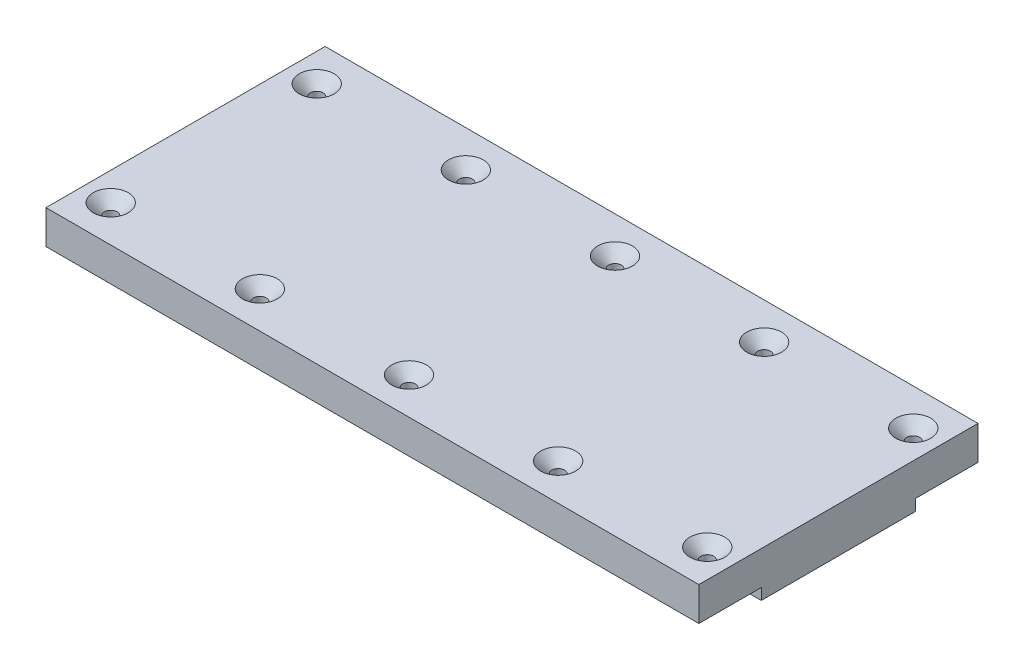
ISO-10303-21;
HEADER;
FILE_DESCRIPTION(('STEP AP214'),'2;1');
FILE_NAME('part.step','',(''),(''),'','','');
FILE_SCHEMA(('AUTOMOTIVE_DESIGN { 1 0 10303 214 1 1 1 1 }'));
ENDSEC;
DATA;
#1=APPLICATION_CONTEXT('core data for automotive mechanical design processes');
#2=APPLICATION_PROTOCOL_DEFINITION('international standard','automotive_design',2000,#1);
#3=PRODUCT_CONTEXT('',#1,'mechanical');
#4=PRODUCT('Part','Part','',(#3));
#5=PRODUCT_RELATED_PRODUCT_CATEGORY('part','',(#4));
#6=PRODUCT_DEFINITION_FORMATION('','',#4);
#7=PRODUCT_DEFINITION_CONTEXT('part definition',#1,'design');
#8=PRODUCT_DEFINITION('design','',#6,#7);
#9=PRODUCT_DEFINITION_SHAPE('','',#8);
#10=(LENGTH_UNIT() NAMED_UNIT(*) SI_UNIT(.MILLI.,.METRE.));
#11=(NAMED_UNIT(*) PLANE_ANGLE_UNIT() SI_UNIT($,.RADIAN.));
#12=(NAMED_UNIT(*) SI_UNIT($,.STERADIAN.) SOLID_ANGLE_UNIT());
#13=UNCERTAINTY_MEASURE_WITH_UNIT(LENGTH_MEASURE(1.E-05),#10,'distance_accuracy_value','');
#14=(GEOMETRIC_REPRESENTATION_CONTEXT(3) GLOBAL_UNCERTAINTY_ASSIGNED_CONTEXT((#13)) GLOBAL_UNIT_ASSIGNED_CONTEXT((#10,
#11,#12)) REPRESENTATION_CONTEXT('',''));
#15=CARTESIAN_POINT('',(0.,0.,0.));
#16=DIRECTION('',(0.,0.,1.));
#17=DIRECTION('',(1.,0.,0.));
#18=AXIS2_PLACEMENT_3D('',#15,#16,#17);
#19=CARTESIAN_POINT('',(580.,10.,68.5));
#20=DIRECTION('',(0.,0.,-1.));
#21=DIRECTION('',(-1.,0.,0.));
#22=AXIS2_PLACEMENT_3D('',#19,#20,#21);
#23=PLANE('',#22);
#24=DIRECTION('',(0.,-1.,0.));
#25=VECTOR('',#24,1.);
#26=CARTESIAN_POINT('',(0.,10.,68.5));
#27=LINE('',#26,#25);
#28=CARTESIAN_POINT('',(0.,10.,68.5));
#29=VERTEX_POINT('',#28);
#30=CARTESIAN_POINT('',(0.,0.,68.5));
#31=VERTEX_POINT('',#30);
#32=EDGE_CURVE('E137',#29,#31,#27,.T.);
#33=ORIENTED_EDGE('',*,*,#32,.T.);
#34=DIRECTION('',(-1.,0.,0.));
#35=VECTOR('',#34,1.);
#36=CARTESIAN_POINT('',(580.,0.,68.5));
#37=LINE('',#36,#35);
#38=CARTESIAN_POINT('',(580.,0.,68.5));
#39=VERTEX_POINT('',#38);
#40=EDGE_CURVE('E169',#39,#31,#37,.T.);
#41=ORIENTED_EDGE('',*,*,#40,.F.);
#42=DIRECTION('',(0.,-1.,0.));
#43=VECTOR('',#42,1.);
#44=CARTESIAN_POINT('',(580.,10.,68.5));
#45=LINE('',#44,#43);
#46=CARTESIAN_POINT('',(580.,10.,68.5));
#47=VERTEX_POINT('',#46);
#48=EDGE_CURVE('E154',#47,#39,#45,.T.);
#49=ORIENTED_EDGE('',*,*,#48,.F.);
#50=DIRECTION('',(-1.,0.,0.));
#51=VECTOR('',#50,1.);
#52=CARTESIAN_POINT('',(580.,10.,68.5));
#53=LINE('',#52,#51);
#54=EDGE_CURVE('E138',#47,#29,#53,.T.);
#55=ORIENTED_EDGE('',*,*,#54,.T.);
#56=EDGE_LOOP('',(#33,#41,#49,#55));
#57=FACE_BOUND('',#56,.T.);
#58=ADVANCED_FACE('F41',(#57),#23,.F.);
#59=CARTESIAN_POINT('',(580.,0.,68.5));
#60=DIRECTION('',(0.,1.,0.));
#61=DIRECTION('',(0.,0.,1.));
#62=AXIS2_PLACEMENT_3D('',#59,#60,#61);
#63=PLANE('',#62);
#64=DIRECTION('',(0.,0.,-1.));
#65=VECTOR('',#64,1.);
#66=CARTESIAN_POINT('',(0.,0.,68.5));
#67=LINE('',#66,#65);
#68=CARTESIAN_POINT('',(0.,0.,-68.5));
#69=VERTEX_POINT('',#68);
#70=EDGE_CURVE('E141',#31,#69,#67,.T.);
#71=ORIENTED_EDGE('',*,*,#70,.T.);
#72=DIRECTION('',(-1.,0.,0.));
#73=VECTOR('',#72,1.);
#74=CARTESIAN_POINT('',(580.,0.,-68.5));
#75=LINE('',#74,#73);
#76=CARTESIAN_POINT('',(580.,0.,-68.5));
#77=VERTEX_POINT('',#76);
#78=EDGE_CURVE('E164',#77,#69,#75,.T.);
#79=ORIENTED_EDGE('',*,*,#78,.F.);
#80=DIRECTION('',(0.,0.,-1.));
#81=VECTOR('',#80,1.);
#82=CARTESIAN_POINT('',(580.,0.,68.5));
#83=LINE('',#82,#81);
#84=EDGE_CURVE('E103',#39,#77,#83,.T.);
#85=ORIENTED_EDGE('',*,*,#84,.F.);
#86=ORIENTED_EDGE('',*,*,#40,.T.);
#87=EDGE_LOOP('',(#71,#79,#85,#86));
#88=FACE_BOUND('',#87,.T.);
#89=ADVANCED_FACE('F257',(#88),#63,.F.);
#90=CARTESIAN_POINT('',(580.,0.,-68.5));
#91=DIRECTION('',(0.,0.,1.));
#92=DIRECTION('',(1.,0.,0.));
#93=AXIS2_PLACEMENT_3D('',#90,#91,#92);
#94=PLANE('',#93);
#95=DIRECTION('',(0.,1.,0.));
#96=VECTOR('',#95,1.);
#97=CARTESIAN_POINT('',(0.,0.,-68.5));
#98=LINE('',#97,#96);
#99=CARTESIAN_POINT('',(0.,10.,-68.5));
#100=VERTEX_POINT('',#99);
#101=EDGE_CURVE('E148',#69,#100,#98,.T.);
#102=ORIENTED_EDGE('',*,*,#101,.T.);
#103=DIRECTION('',(-1.,0.,0.));
#104=VECTOR('',#103,1.);
#105=CARTESIAN_POINT('',(580.,10.,-68.5));
#106=LINE('',#105,#104);
#107=CARTESIAN_POINT('',(580.,10.,-68.5));
#108=VERTEX_POINT('',#107);
#109=EDGE_CURVE('E165',#108,#100,#106,.T.);
#110=ORIENTED_EDGE('',*,*,#109,.F.);
#111=DIRECTION('',(0.,1.,0.));
#112=VECTOR('',#111,1.);
#113=CARTESIAN_POINT('',(580.,0.,-68.5));
#114=LINE('',#113,#112);
#115=EDGE_CURVE('E351',#77,#108,#114,.T.);
#116=ORIENTED_EDGE('',*,*,#115,.F.);
#117=ORIENTED_EDGE('',*,*,#78,.T.);
#118=EDGE_LOOP('',(#102,#110,#116,#117));
#119=FACE_BOUND('',#118,.T.);
#120=ADVANCED_FACE('F266',(#119),#94,.F.);
#121=CARTESIAN_POINT('',(580.,10.,-68.5));
#122=DIRECTION('',(0.,1.,0.));
#123=DIRECTION('',(0.,0.,1.));
#124=AXIS2_PLACEMENT_3D('',#121,#122,#123);
#125=PLANE('',#124);
#126=CARTESIAN_POINT('',(25.,10.,-91.5));
#127=DIRECTION('',(0.,1.,0.));
#128=DIRECTION('',(0.,0.,1.));
#129=AXIS2_PLACEMENT_3D('',#126,#127,#128);
#130=CIRCLE('',#129,5.7);
#131=CARTESIAN_POINT('',(25.,10.,-85.8));
#132=VERTEX_POINT('',#131);
#133=EDGE_CURVE('E145',#132,#132,#130,.T.);
#134=ORIENTED_EDGE('',*,*,#133,.T.);
#135=EDGE_LOOP('',(#134));
#136=FACE_BOUND('',#135,.T.);
#137=CARTESIAN_POINT('',(157.5,10.,-91.5));
#138=DIRECTION('',(0.,1.,0.));
#139=DIRECTION('',(0.,0.,1.));
#140=AXIS2_PLACEMENT_3D('',#137,#138,#139);
#141=CIRCLE('',#140,5.70000000000001);
#142=CARTESIAN_POINT('',(157.5,10.,-85.8));
#143=VERTEX_POINT('',#142);
#144=EDGE_CURVE('E344',#143,#143,#141,.T.);
#145=ORIENTED_EDGE('',*,*,#144,.T.);
#146=EDGE_LOOP('',(#145));
#147=FACE_BOUND('',#146,.T.);
#148=CARTESIAN_POINT('',(290.,10.,-91.5));
#149=DIRECTION('',(0.,1.,0.));
#150=DIRECTION('',(0.,0.,1.));
#151=AXIS2_PLACEMENT_3D('',#148,#149,#150);
#152=CIRCLE('',#151,5.7);
#153=CARTESIAN_POINT('',(290.,10.,-85.8));
#154=VERTEX_POINT('',#153);
#155=EDGE_CURVE('E343',#154,#154,#152,.T.);
#156=ORIENTED_EDGE('',*,*,#155,.T.);
#157=EDGE_LOOP('',(#156));
#158=FACE_BOUND('',#157,.T.);
#159=CARTESIAN_POINT('',(422.5,10.,-91.5));
#160=DIRECTION('',(0.,1.,0.));
#161=DIRECTION('',(0.,0.,1.));
#162=AXIS2_PLACEMENT_3D('',#159,#160,#161);
#163=CIRCLE('',#162,5.7);
#164=CARTESIAN_POINT('',(422.5,10.,-85.8));
#165=VERTEX_POINT('',#164);
#166=EDGE_CURVE('E339',#165,#165,#163,.T.);
#167=ORIENTED_EDGE('',*,*,#166,.T.);
#168=EDGE_LOOP('',(#167));
#169=FACE_BOUND('',#168,.T.);
#170=CARTESIAN_POINT('',(555.,10.,-91.5));
#171=DIRECTION('',(0.,1.,0.));
#172=DIRECTION('',(0.,0.,1.));
#173=AXIS2_PLACEMENT_3D('',#170,#171,#172);
#174=CIRCLE('',#173,5.70000000000006);
#175=CARTESIAN_POINT('',(555.,10.,-85.7999999999999));
#176=VERTEX_POINT('',#175);
#177=EDGE_CURVE('E187',#176,#176,#174,.T.);
#178=ORIENTED_EDGE('',*,*,#177,.T.);
#179=EDGE_LOOP('',(#178));
#180=FACE_BOUND('',#179,.T.);
#181=DIRECTION('',(0.,0.,-1.));
#182=VECTOR('',#181,1.);
#183=CARTESIAN_POINT('',(0.,10.,-68.5));
#184=LINE('',#183,#182);
#185=CARTESIAN_POINT('',(0.,10.,-124.));
#186=VERTEX_POINT('',#185);
#187=EDGE_CURVE('E146',#100,#186,#184,.T.);
#188=ORIENTED_EDGE('',*,*,#187,.T.);
#189=DIRECTION('',(-1.,0.,0.));
#190=VECTOR('',#189,1.);
#191=CARTESIAN_POINT('',(580.,10.,-124.));
#192=LINE('',#191,#190);
#193=CARTESIAN_POINT('',(580.,10.,-124.));
#194=VERTEX_POINT('',#193);
#195=EDGE_CURVE('E157',#194,#186,#192,.T.);
#196=ORIENTED_EDGE('',*,*,#195,.F.);
#197=DIRECTION('',(0.,0.,-1.));
#198=VECTOR('',#197,1.);
#199=CARTESIAN_POINT('',(580.,10.,-68.5));
#200=LINE('',#199,#198);
#201=EDGE_CURVE('E360',#108,#194,#200,.T.);
#202=ORIENTED_EDGE('',*,*,#201,.F.);
#203=ORIENTED_EDGE('',*,*,#109,.T.);
#204=EDGE_LOOP('',(#188,#196,#202,#203));
#205=FACE_BOUND('',#204,.T.);
#206=ADVANCED_FACE('F361',(#136,#147,#158,#169,#180,#205),#125,.F.);
#207=CARTESIAN_POINT('',(580.,10.,-124.));
#208=DIRECTION('',(0.,0.,1.));
#209=DIRECTION('',(1.,0.,0.));
#210=AXIS2_PLACEMENT_3D('',#207,#208,#209);
#211=PLANE('',#210);
#212=DIRECTION('',(0.,1.,0.));
#213=VECTOR('',#212,1.);
#214=CARTESIAN_POINT('',(0.,10.,-124.));
#215=LINE('',#214,#213);
#216=CARTESIAN_POINT('',(0.,40.,-124.));
#217=VERTEX_POINT('',#216);
#218=EDGE_CURVE('E147',#186,#217,#215,.T.);
#219=ORIENTED_EDGE('',*,*,#218,.T.);
#220=DIRECTION('',(-1.,0.,0.));
#221=VECTOR('',#220,1.);
#222=CARTESIAN_POINT('',(580.,40.,-124.));
#223=LINE('',#222,#221);
#224=CARTESIAN_POINT('',(580.,40.,-124.));
#225=VERTEX_POINT('',#224);
#226=EDGE_CURVE('E132',#225,#217,#223,.T.);
#227=ORIENTED_EDGE('',*,*,#226,.F.);
#228=DIRECTION('',(0.,1.,0.));
#229=VECTOR('',#228,1.);
#230=CARTESIAN_POINT('',(580.,10.,-124.));
#231=LINE('',#230,#229);
#232=EDGE_CURVE('E125',#194,#225,#231,.T.);
#233=ORIENTED_EDGE('',*,*,#232,.F.);
#234=ORIENTED_EDGE('',*,*,#195,.T.);
#235=EDGE_LOOP('',(#219,#227,#233,#234));
#236=FACE_BOUND('',#235,.T.);
#237=ADVANCED_FACE('F370',(#236),#211,.F.);
#238=CARTESIAN_POINT('',(580.,40.,-124.));
#239=DIRECTION('',(0.,-1.,0.));
#240=DIRECTION('',(0.,0.,-1.));
#241=AXIS2_PLACEMENT_3D('',#238,#239,#240);
#242=PLANE('',#241);
#243=CARTESIAN_POINT('',(422.5,40.,91.5));
#244=DIRECTION('',(0.,-1.,0.));
#245=DIRECTION('',(0.,0.,-1.));
#246=AXIS2_PLACEMENT_3D('',#243,#244,#245);
#247=CIRCLE('',#246,15.5000000000002);
#248=CARTESIAN_POINT('',(422.5,40.,75.9999999999998));
#249=VERTEX_POINT('',#248);
#250=EDGE_CURVE('E216',#249,#249,#247,.T.);
#251=ORIENTED_EDGE('',*,*,#250,.T.);
#252=EDGE_LOOP('',(#251));
#253=FACE_BOUND('',#252,.T.);
#254=CARTESIAN_POINT('',(25.,40.,91.5));
#255=DIRECTION('',(0.,-1.,0.));
#256=DIRECTION('',(0.,0.,-1.));
#257=AXIS2_PLACEMENT_3D('',#254,#255,#256);
#258=CIRCLE('',#257,15.5000000000002);
#259=CARTESIAN_POINT('',(25.,40.,75.9999999999998));
#260=VERTEX_POINT('',#259);
#261=EDGE_CURVE('E213',#260,#260,#258,.T.);
#262=ORIENTED_EDGE('',*,*,#261,.T.);
#263=EDGE_LOOP('',(#262));
#264=FACE_BOUND('',#263,.T.);
#265=CARTESIAN_POINT('',(157.5,40.,91.5));
#266=DIRECTION('',(0.,-1.,0.));
#267=DIRECTION('',(0.,0.,-1.));
#268=AXIS2_PLACEMENT_3D('',#265,#266,#267);
#269=CIRCLE('',#268,15.5000000000002);
#270=CARTESIAN_POINT('',(157.5,40.,75.9999999999998));
#271=VERTEX_POINT('',#270);
#272=EDGE_CURVE('E209',#271,#271,#269,.T.);
#273=ORIENTED_EDGE('',*,*,#272,.T.);
#274=EDGE_LOOP('',(#273));
#275=FACE_BOUND('',#274,.T.);
#276=CARTESIAN_POINT('',(290.,40.,91.5));
#277=DIRECTION('',(0.,-1.,0.));
#278=DIRECTION('',(0.,0.,-1.));
#279=AXIS2_PLACEMENT_3D('',#276,#277,#278);
#280=CIRCLE('',#279,15.5000000000002);
#281=CARTESIAN_POINT('',(290.,40.,75.9999999999998));
#282=VERTEX_POINT('',#281);
#283=EDGE_CURVE('E210',#282,#282,#280,.T.);
#284=ORIENTED_EDGE('',*,*,#283,.T.);
#285=EDGE_LOOP('',(#284));
#286=FACE_BOUND('',#285,.T.);
#287=CARTESIAN_POINT('',(555.,40.,91.5));
#288=DIRECTION('',(0.,-1.,0.));
#289=DIRECTION('',(0.,0.,-1.));
#290=AXIS2_PLACEMENT_3D('',#287,#288,#289);
#291=CIRCLE('',#290,15.5000000000002);
#292=CARTESIAN_POINT('',(555.,40.,75.9999999999998));
#293=VERTEX_POINT('',#292);
#294=EDGE_CURVE('E204',#293,#293,#291,.T.);
#295=ORIENTED_EDGE('',*,*,#294,.T.);
#296=EDGE_LOOP('',(#295));
#297=FACE_BOUND('',#296,.T.);
#298=CARTESIAN_POINT('',(555.,40.,-91.5));
#299=DIRECTION('',(0.,-1.,0.));
#300=DIRECTION('',(0.,0.,-1.));
#301=AXIS2_PLACEMENT_3D('',#298,#299,#300);
#302=CIRCLE('',#301,15.5000000000002);
#303=CARTESIAN_POINT('',(555.,40.,-107.));
#304=VERTEX_POINT('',#303);
#305=EDGE_CURVE('E203',#304,#304,#302,.T.);
#306=ORIENTED_EDGE('',*,*,#305,.T.);
#307=EDGE_LOOP('',(#306));
#308=FACE_BOUND('',#307,.T.);
#309=CARTESIAN_POINT('',(422.5,40.,-91.5));
#310=DIRECTION('',(0.,-1.,0.));
#311=DIRECTION('',(0.,0.,-1.));
#312=AXIS2_PLACEMENT_3D('',#309,#310,#311);
#313=CIRCLE('',#312,15.5000000000002);
#314=CARTESIAN_POINT('',(422.5,40.,-107.));
#315=VERTEX_POINT('',#314);
#316=EDGE_CURVE('E196',#315,#315,#313,.T.);
#317=ORIENTED_EDGE('',*,*,#316,.T.);
#318=EDGE_LOOP('',(#317));
#319=FACE_BOUND('',#318,.T.);
#320=CARTESIAN_POINT('',(290.,40.,-91.5));
#321=DIRECTION('',(0.,-1.,0.));
#322=DIRECTION('',(0.,0.,-1.));
#323=AXIS2_PLACEMENT_3D('',#320,#321,#322);
#324=CIRCLE('',#323,15.5000000000002);
#325=CARTESIAN_POINT('',(290.,40.,-107.));
#326=VERTEX_POINT('',#325);
#327=EDGE_CURVE('E192',#326,#326,#324,.T.);
#328=ORIENTED_EDGE('',*,*,#327,.T.);
#329=EDGE_LOOP('',(#328));
#330=FACE_BOUND('',#329,.T.);
#331=CARTESIAN_POINT('',(157.5,40.,-91.5));
#332=DIRECTION('',(0.,-1.,0.));
#333=DIRECTION('',(0.,0.,-1.));
#334=AXIS2_PLACEMENT_3D('',#331,#332,#333);
#335=CIRCLE('',#334,15.5000000000002);
#336=CARTESIAN_POINT('',(157.5,40.,-107.));
#337=VERTEX_POINT('',#336);
#338=EDGE_CURVE('E195',#337,#337,#335,.T.);
#339=ORIENTED_EDGE('',*,*,#338,.T.);
#340=EDGE_LOOP('',(#339));
#341=FACE_BOUND('',#340,.T.);
#342=CARTESIAN_POINT('',(25.,40.,-91.5));
#343=DIRECTION('',(0.,-1.,0.));
#344=DIRECTION('',(0.,0.,-1.));
#345=AXIS2_PLACEMENT_3D('',#342,#343,#344);
#346=CIRCLE('',#345,15.5000000000002);
#347=CARTESIAN_POINT('',(25.,40.,-107.));
#348=VERTEX_POINT('',#347);
#349=EDGE_CURVE('E189',#348,#348,#346,.T.);
#350=ORIENTED_EDGE('',*,*,#349,.T.);
#351=EDGE_LOOP('',(#350));
#352=FACE_BOUND('',#351,.T.);
#353=DIRECTION('',(0.,0.,1.));
#354=VECTOR('',#353,1.);
#355=CARTESIAN_POINT('',(0.,40.,-124.));
#356=LINE('',#355,#354);
#357=CARTESIAN_POINT('',(0.,40.,124.));
#358=VERTEX_POINT('',#357);
#359=EDGE_CURVE('E128',#217,#358,#356,.T.);
#360=ORIENTED_EDGE('',*,*,#359,.T.);
#361=DIRECTION('',(-1.,0.,0.));
#362=VECTOR('',#361,1.);
#363=CARTESIAN_POINT('',(580.,40.,124.));
#364=LINE('',#363,#362);
#365=CARTESIAN_POINT('',(580.,40.,124.));
#366=VERTEX_POINT('',#365);
#367=EDGE_CURVE('E130',#366,#358,#364,.T.);
#368=ORIENTED_EDGE('',*,*,#367,.F.);
#369=DIRECTION('',(0.,0.,1.));
#370=VECTOR('',#369,1.);
#371=CARTESIAN_POINT('',(580.,40.,-124.));
#372=LINE('',#371,#370);
#373=EDGE_CURVE('E117',#225,#366,#372,.T.);
#374=ORIENTED_EDGE('',*,*,#373,.F.);
#375=ORIENTED_EDGE('',*,*,#226,.T.);
#376=EDGE_LOOP('',(#360,#368,#374,#375));
#377=FACE_BOUND('',#376,.T.);
#378=ADVANCED_FACE('F126',(#253,#264,#275,#286,#297,#308,#319,#330,#341,#352,#377),#242,.F.);
#379=CARTESIAN_POINT('',(580.,40.,124.));
#380=DIRECTION('',(0.,0.,-1.));
#381=DIRECTION('',(-1.,0.,0.));
#382=AXIS2_PLACEMENT_3D('',#379,#380,#381);
#383=PLANE('',#382);
#384=DIRECTION('',(0.,-1.,0.));
#385=VECTOR('',#384,1.);
#386=CARTESIAN_POINT('',(0.,40.,124.));
#387=LINE('',#386,#385);
#388=CARTESIAN_POINT('',(0.,10.,124.));
#389=VERTEX_POINT('',#388);
#390=EDGE_CURVE('E86',#358,#389,#387,.T.);
#391=ORIENTED_EDGE('',*,*,#390,.T.);
#392=DIRECTION('',(-1.,0.,0.));
#393=VECTOR('',#392,1.);
#394=CARTESIAN_POINT('',(580.,10.,124.));
#395=LINE('',#394,#393);
#396=CARTESIAN_POINT('',(580.,10.,124.));
#397=VERTEX_POINT('',#396);
#398=EDGE_CURVE('E135',#397,#389,#395,.T.);
#399=ORIENTED_EDGE('',*,*,#398,.F.);
#400=DIRECTION('',(0.,-1.,0.));
#401=VECTOR('',#400,1.);
#402=CARTESIAN_POINT('',(580.,40.,124.));
#403=LINE('',#402,#401);
#404=EDGE_CURVE('E116',#366,#397,#403,.T.);
#405=ORIENTED_EDGE('',*,*,#404,.F.);
#406=ORIENTED_EDGE('',*,*,#367,.T.);
#407=EDGE_LOOP('',(#391,#399,#405,#406));
#408=FACE_BOUND('',#407,.T.);
#409=ADVANCED_FACE('F134',(#408),#383,.F.);
#410=CARTESIAN_POINT('',(580.,10.,124.));
#411=DIRECTION('',(0.,1.,0.));
#412=DIRECTION('',(0.,0.,1.));
#413=AXIS2_PLACEMENT_3D('',#410,#411,#412);
#414=PLANE('',#413);
#415=CARTESIAN_POINT('',(157.5,10.,91.5));
#416=DIRECTION('',(0.,1.,0.));
#417=DIRECTION('',(0.,0.,1.));
#418=AXIS2_PLACEMENT_3D('',#415,#416,#417);
#419=CIRCLE('',#418,5.70000000000001);
#420=CARTESIAN_POINT('',(157.5,10.,97.2));
#421=VERTEX_POINT('',#420);
#422=EDGE_CURVE('E181',#421,#421,#419,.T.);
#423=ORIENTED_EDGE('',*,*,#422,.T.);
#424=EDGE_LOOP('',(#423));
#425=FACE_BOUND('',#424,.T.);
#426=CARTESIAN_POINT('',(422.5,10.,91.5));
#427=DIRECTION('',(0.,1.,0.));
#428=DIRECTION('',(0.,0.,1.));
#429=AXIS2_PLACEMENT_3D('',#426,#427,#428);
#430=CIRCLE('',#429,5.7);
#431=CARTESIAN_POINT('',(422.5,10.,97.2));
#432=VERTEX_POINT('',#431);
#433=EDGE_CURVE('E177',#432,#432,#430,.T.);
#434=ORIENTED_EDGE('',*,*,#433,.T.);
#435=EDGE_LOOP('',(#434));
#436=FACE_BOUND('',#435,.T.);
#437=CARTESIAN_POINT('',(555.,10.,91.5));
#438=DIRECTION('',(0.,1.,0.));
#439=DIRECTION('',(0.,0.,1.));
#440=AXIS2_PLACEMENT_3D('',#437,#438,#439);
#441=CIRCLE('',#440,5.70000000000006);
#442=CARTESIAN_POINT('',(555.,10.,97.2000000000001));
#443=VERTEX_POINT('',#442);
#444=EDGE_CURVE('E180',#443,#443,#441,.T.);
#445=ORIENTED_EDGE('',*,*,#444,.T.);
#446=EDGE_LOOP('',(#445));
#447=FACE_BOUND('',#446,.T.);
#448=CARTESIAN_POINT('',(290.,10.,91.5));
#449=DIRECTION('',(0.,1.,0.));
#450=DIRECTION('',(0.,0.,1.));
#451=AXIS2_PLACEMENT_3D('',#448,#449,#450);
#452=CIRCLE('',#451,5.7);
#453=CARTESIAN_POINT('',(290.,10.,97.2));
#454=VERTEX_POINT('',#453);
#455=EDGE_CURVE('E174',#454,#454,#452,.T.);
#456=ORIENTED_EDGE('',*,*,#455,.T.);
#457=EDGE_LOOP('',(#456));
#458=FACE_BOUND('',#457,.T.);
#459=CARTESIAN_POINT('',(25.,10.,91.5));
#460=DIRECTION('',(0.,1.,0.));
#461=DIRECTION('',(0.,0.,1.));
#462=AXIS2_PLACEMENT_3D('',#459,#460,#461);
#463=CIRCLE('',#462,5.7);
#464=CARTESIAN_POINT('',(25.,10.,97.2));
#465=VERTEX_POINT('',#464);
#466=EDGE_CURVE('E172',#465,#465,#463,.T.);
#467=ORIENTED_EDGE('',*,*,#466,.T.);
#468=EDGE_LOOP('',(#467));
#469=FACE_BOUND('',#468,.T.);
#470=DIRECTION('',(0.,0.,-1.));
#471=VECTOR('',#470,1.);
#472=CARTESIAN_POINT('',(0.,10.,124.));
#473=LINE('',#472,#471);
#474=EDGE_CURVE('E94',#389,#29,#473,.T.);
#475=ORIENTED_EDGE('',*,*,#474,.T.);
#476=ORIENTED_EDGE('',*,*,#54,.F.);
#477=DIRECTION('',(0.,0.,-1.));
#478=VECTOR('',#477,1.);
#479=CARTESIAN_POINT('',(580.,10.,124.));
#480=LINE('',#479,#478);
#481=EDGE_CURVE('E56',#397,#47,#480,.T.);
#482=ORIENTED_EDGE('',*,*,#481,.F.);
#483=ORIENTED_EDGE('',*,*,#398,.T.);
#484=EDGE_LOOP('',(#475,#476,#482,#483));
#485=FACE_BOUND('',#484,.T.);
#486=ADVANCED_FACE('F372',(#425,#436,#447,#458,#469,#485),#414,.F.);
#487=CARTESIAN_POINT('',(580.,0.,0.));
#488=DIRECTION('',(1.,0.,0.));
#489=DIRECTION('',(0.,0.,-1.));
#490=AXIS2_PLACEMENT_3D('',#487,#488,#489);
#491=PLANE('',#490);
#492=ORIENTED_EDGE('',*,*,#48,.T.);
#493=ORIENTED_EDGE('',*,*,#84,.T.);
#494=ORIENTED_EDGE('',*,*,#115,.T.);
#495=ORIENTED_EDGE('',*,*,#201,.T.);
#496=ORIENTED_EDGE('',*,*,#232,.T.);
#497=ORIENTED_EDGE('',*,*,#373,.T.);
#498=ORIENTED_EDGE('',*,*,#404,.T.);
#499=ORIENTED_EDGE('',*,*,#481,.T.);
#500=EDGE_LOOP('',(#492,#493,#494,#495,#496,#497,#498,#499));
#501=FACE_BOUND('',#500,.T.);
#502=ADVANCED_FACE('F118',(#501),#491,.T.);
#503=CARTESIAN_POINT('',(0.,0.,0.));
#504=DIRECTION('',(1.,0.,0.));
#505=DIRECTION('',(0.,0.,-1.));
#506=AXIS2_PLACEMENT_3D('',#503,#504,#505);
#507=PLANE('',#506);
#508=ORIENTED_EDGE('',*,*,#32,.F.);
#509=ORIENTED_EDGE('',*,*,#474,.F.);
#510=ORIENTED_EDGE('',*,*,#390,.F.);
#511=ORIENTED_EDGE('',*,*,#359,.F.);
#512=ORIENTED_EDGE('',*,*,#218,.F.);
#513=ORIENTED_EDGE('',*,*,#187,.F.);
#514=ORIENTED_EDGE('',*,*,#101,.F.);
#515=ORIENTED_EDGE('',*,*,#70,.F.);
#516=EDGE_LOOP('',(#508,#509,#510,#511,#512,#513,#514,#515));
#517=FACE_BOUND('',#516,.T.);
#518=ADVANCED_FACE('F367',(#517),#507,.F.);
#519=CARTESIAN_POINT('',(25.,-540.,91.5));
#520=DIRECTION('',(0.,1.,0.));
#521=DIRECTION('',(0.,0.,1.));
#522=AXIS2_PLACEMENT_3D('',#519,#520,#521);
#523=CYLINDRICAL_SURFACE('',#522,5.7);
#524=CARTESIAN_POINT('',(25.,30.1999999999998,91.5));
#525=DIRECTION('',(0.,-1.,0.));
#526=DIRECTION('',(0.,0.,-1.));
#527=AXIS2_PLACEMENT_3D('',#524,#525,#526);
#528=CIRCLE('',#527,5.7);
#529=CARTESIAN_POINT('',(25.,30.1999999999998,85.8));
#530=VERTEX_POINT('',#529);
#531=EDGE_CURVE('E218',#530,#530,#528,.F.);
#532=ORIENTED_EDGE('',*,*,#531,.T.);
#533=EDGE_LOOP('',(#532));
#534=FACE_BOUND('',#533,.T.);
#535=ORIENTED_EDGE('',*,*,#466,.F.);
#536=EDGE_LOOP('',(#535));
#537=FACE_BOUND('',#536,.T.);
#538=ADVANCED_FACE('F421',(#534,#537),#523,.F.);
#539=CARTESIAN_POINT('',(290.,-540.,91.5));
#540=DIRECTION('',(0.,1.,0.));
#541=DIRECTION('',(0.,0.,1.));
#542=AXIS2_PLACEMENT_3D('',#539,#540,#541);
#543=CYLINDRICAL_SURFACE('',#542,5.7);
#544=CARTESIAN_POINT('',(290.,30.1999999999998,91.5));
#545=DIRECTION('',(0.,-1.,0.));
#546=DIRECTION('',(0.,0.,-1.));
#547=AXIS2_PLACEMENT_3D('',#544,#545,#546);
#548=CIRCLE('',#547,5.7);
#549=CARTESIAN_POINT('',(290.,30.1999999999998,85.8));
#550=VERTEX_POINT('',#549);
#551=EDGE_CURVE('E223',#550,#550,#548,.F.);
#552=ORIENTED_EDGE('',*,*,#551,.T.);
#553=EDGE_LOOP('',(#552));
#554=FACE_BOUND('',#553,.T.);
#555=ORIENTED_EDGE('',*,*,#455,.F.);
#556=EDGE_LOOP('',(#555));
#557=FACE_BOUND('',#556,.T.);
#558=ADVANCED_FACE('F453',(#554,#557),#543,.F.);
#559=CARTESIAN_POINT('',(555.,-540.,91.5));
#560=DIRECTION('',(0.,1.,0.));
#561=DIRECTION('',(0.,0.,1.));
#562=AXIS2_PLACEMENT_3D('',#559,#560,#561);
#563=CYLINDRICAL_SURFACE('',#562,5.70000000000006);
#564=CARTESIAN_POINT('',(555.,30.1999999999999,91.5));
#565=DIRECTION('',(0.,-1.,0.));
#566=DIRECTION('',(0.,0.,-1.));
#567=AXIS2_PLACEMENT_3D('',#564,#565,#566);
#568=CIRCLE('',#567,5.70000000000006);
#569=CARTESIAN_POINT('',(555.,30.1999999999999,85.7999999999999));
#570=VERTEX_POINT('',#569);
#571=EDGE_CURVE('E228',#570,#570,#568,.F.);
#572=ORIENTED_EDGE('',*,*,#571,.T.);
#573=EDGE_LOOP('',(#572));
#574=FACE_BOUND('',#573,.T.);
#575=ORIENTED_EDGE('',*,*,#444,.F.);
#576=EDGE_LOOP('',(#575));
#577=FACE_BOUND('',#576,.T.);
#578=ADVANCED_FACE('F458',(#574,#577),#563,.F.);
#579=CARTESIAN_POINT('',(422.5,-540.,91.5));
#580=DIRECTION('',(0.,1.,0.));
#581=DIRECTION('',(0.,0.,1.));
#582=AXIS2_PLACEMENT_3D('',#579,#580,#581);
#583=CYLINDRICAL_SURFACE('',#582,5.7);
#584=CARTESIAN_POINT('',(422.5,30.1999999999998,91.5));
#585=DIRECTION('',(0.,-1.,0.));
#586=DIRECTION('',(0.,0.,-1.));
#587=AXIS2_PLACEMENT_3D('',#584,#585,#586);
#588=CIRCLE('',#587,5.7);
#589=CARTESIAN_POINT('',(422.5,30.1999999999998,85.8));
#590=VERTEX_POINT('',#589);
#591=EDGE_CURVE('E168',#590,#590,#588,.F.);
#592=ORIENTED_EDGE('',*,*,#591,.T.);
#593=EDGE_LOOP('',(#592));
#594=FACE_BOUND('',#593,.T.);
#595=ORIENTED_EDGE('',*,*,#433,.F.);
#596=EDGE_LOOP('',(#595));
#597=FACE_BOUND('',#596,.T.);
#598=ADVANCED_FACE('F469',(#594,#597),#583,.F.);
#599=CARTESIAN_POINT('',(157.5,-540.,91.5));
#600=DIRECTION('',(0.,1.,0.));
#601=DIRECTION('',(0.,0.,1.));
#602=AXIS2_PLACEMENT_3D('',#599,#600,#601);
#603=CYLINDRICAL_SURFACE('',#602,5.70000000000001);
#604=CARTESIAN_POINT('',(157.5,30.1999999999998,91.5));
#605=DIRECTION('',(0.,-1.,0.));
#606=DIRECTION('',(0.,0.,-1.));
#607=AXIS2_PLACEMENT_3D('',#604,#605,#606);
#608=CIRCLE('',#607,5.70000000000001);
#609=CARTESIAN_POINT('',(157.5,30.1999999999998,85.8));
#610=VERTEX_POINT('',#609);
#611=EDGE_CURVE('E225',#610,#610,#608,.F.);
#612=ORIENTED_EDGE('',*,*,#611,.T.);
#613=EDGE_LOOP('',(#612));
#614=FACE_BOUND('',#613,.T.);
#615=ORIENTED_EDGE('',*,*,#422,.F.);
#616=EDGE_LOOP('',(#615));
#617=FACE_BOUND('',#616,.T.);
#618=ADVANCED_FACE('F476',(#614,#617),#603,.F.);
#619=CARTESIAN_POINT('',(555.,-540.,-91.5));
#620=DIRECTION('',(0.,1.,0.));
#621=DIRECTION('',(0.,0.,1.));
#622=AXIS2_PLACEMENT_3D('',#619,#620,#621);
#623=CYLINDRICAL_SURFACE('',#622,5.70000000000006);
#624=CARTESIAN_POINT('',(555.,30.1999999999999,-91.5));
#625=DIRECTION('',(0.,-1.,0.));
#626=DIRECTION('',(0.,0.,-1.));
#627=AXIS2_PLACEMENT_3D('',#624,#625,#626);
#628=CIRCLE('',#627,5.70000000000006);
#629=CARTESIAN_POINT('',(555.,30.1999999999999,-97.2000000000001));
#630=VERTEX_POINT('',#629);
#631=EDGE_CURVE('E233',#630,#630,#628,.F.);
#632=ORIENTED_EDGE('',*,*,#631,.T.);
#633=EDGE_LOOP('',(#632));
#634=FACE_BOUND('',#633,.T.);
#635=ORIENTED_EDGE('',*,*,#177,.F.);
#636=EDGE_LOOP('',(#635));
#637=FACE_BOUND('',#636,.T.);
#638=ADVANCED_FACE('F333',(#634,#637),#623,.F.);
#639=CARTESIAN_POINT('',(422.5,-540.,-91.5));
#640=DIRECTION('',(0.,1.,0.));
#641=DIRECTION('',(0.,0.,1.));
#642=AXIS2_PLACEMENT_3D('',#639,#640,#641);
#643=CYLINDRICAL_SURFACE('',#642,5.7);
#644=CARTESIAN_POINT('',(422.5,30.1999999999998,-91.5));
#645=DIRECTION('',(0.,-1.,0.));
#646=DIRECTION('',(0.,0.,-1.));
#647=AXIS2_PLACEMENT_3D('',#644,#645,#646);
#648=CIRCLE('',#647,5.7);
#649=CARTESIAN_POINT('',(422.5,30.1999999999998,-97.2));
#650=VERTEX_POINT('',#649);
#651=EDGE_CURVE('E234',#650,#650,#648,.F.);
#652=ORIENTED_EDGE('',*,*,#651,.T.);
#653=EDGE_LOOP('',(#652));
#654=FACE_BOUND('',#653,.T.);
#655=ORIENTED_EDGE('',*,*,#166,.F.);
#656=EDGE_LOOP('',(#655));
#657=FACE_BOUND('',#656,.T.);
#658=ADVANCED_FACE('F332',(#654,#657),#643,.F.);
#659=CARTESIAN_POINT('',(290.,-540.,-91.5));
#660=DIRECTION('',(0.,1.,0.));
#661=DIRECTION('',(0.,0.,1.));
#662=AXIS2_PLACEMENT_3D('',#659,#660,#661);
#663=CYLINDRICAL_SURFACE('',#662,5.7);
#664=CARTESIAN_POINT('',(290.,30.1999999999998,-91.5));
#665=DIRECTION('',(0.,-1.,0.));
#666=DIRECTION('',(0.,0.,-1.));
#667=AXIS2_PLACEMENT_3D('',#664,#665,#666);
#668=CIRCLE('',#667,5.7);
#669=CARTESIAN_POINT('',(290.,30.1999999999998,-97.2));
#670=VERTEX_POINT('',#669);
#671=EDGE_CURVE('E240',#670,#670,#668,.F.);
#672=ORIENTED_EDGE('',*,*,#671,.T.);
#673=EDGE_LOOP('',(#672));
#674=FACE_BOUND('',#673,.T.);
#675=ORIENTED_EDGE('',*,*,#155,.F.);
#676=EDGE_LOOP('',(#675));
#677=FACE_BOUND('',#676,.T.);
#678=ADVANCED_FACE('F331',(#674,#677),#663,.F.);
#679=CARTESIAN_POINT('',(157.5,-540.,-91.5));
#680=DIRECTION('',(0.,1.,0.));
#681=DIRECTION('',(0.,0.,1.));
#682=AXIS2_PLACEMENT_3D('',#679,#680,#681);
#683=CYLINDRICAL_SURFACE('',#682,5.70000000000001);
#684=CARTESIAN_POINT('',(157.5,30.1999999999998,-91.5));
#685=DIRECTION('',(0.,-1.,0.));
#686=DIRECTION('',(0.,0.,-1.));
#687=AXIS2_PLACEMENT_3D('',#684,#685,#686);
#688=CIRCLE('',#687,5.70000000000001);
#689=CARTESIAN_POINT('',(157.5,30.1999999999998,-97.2));
#690=VERTEX_POINT('',#689);
#691=EDGE_CURVE('E51',#690,#690,#688,.F.);
#692=ORIENTED_EDGE('',*,*,#691,.T.);
#693=EDGE_LOOP('',(#692));
#694=FACE_BOUND('',#693,.T.);
#695=ORIENTED_EDGE('',*,*,#144,.F.);
#696=EDGE_LOOP('',(#695));
#697=FACE_BOUND('',#696,.T.);
#698=ADVANCED_FACE('F245',(#694,#697),#683,.F.);
#699=CARTESIAN_POINT('',(25.,-540.,-91.5));
#700=DIRECTION('',(0.,1.,0.));
#701=DIRECTION('',(0.,0.,1.));
#702=AXIS2_PLACEMENT_3D('',#699,#700,#701);
#703=CYLINDRICAL_SURFACE('',#702,5.7);
#704=CARTESIAN_POINT('',(25.,30.1999999999998,-91.5));
#705=DIRECTION('',(0.,-1.,0.));
#706=DIRECTION('',(0.,0.,-1.));
#707=AXIS2_PLACEMENT_3D('',#704,#705,#706);
#708=CIRCLE('',#707,5.7);
#709=CARTESIAN_POINT('',(25.,30.1999999999998,-97.2));
#710=VERTEX_POINT('',#709);
#711=EDGE_CURVE('E11',#710,#710,#708,.F.);
#712=ORIENTED_EDGE('',*,*,#711,.T.);
#713=EDGE_LOOP('',(#712));
#714=FACE_BOUND('',#713,.T.);
#715=ORIENTED_EDGE('',*,*,#133,.F.);
#716=EDGE_LOOP('',(#715));
#717=FACE_BOUND('',#716,.T.);
#718=ADVANCED_FACE('F279',(#714,#717),#703,.F.);
#719=CARTESIAN_POINT('',(422.5,30.1999999999998,91.5));
#720=DIRECTION('',(0.,1.,0.));
#721=DIRECTION('',(0.,0.,1.));
#722=AXIS2_PLACEMENT_3D('',#719,#720,#721);
#723=CONICAL_SURFACE('',#722,5.7,0.78539816339745);
#724=ORIENTED_EDGE('',*,*,#250,.F.);
#725=EDGE_LOOP('',(#724));
#726=FACE_BOUND('',#725,.T.);
#727=ORIENTED_EDGE('',*,*,#591,.F.);
#728=EDGE_LOOP('',(#727));
#729=FACE_BOUND('',#728,.T.);
#730=ADVANCED_FACE('F271',(#726,#729),#723,.F.);
#731=CARTESIAN_POINT('',(25.,30.1999999999998,91.5));
#732=DIRECTION('',(0.,1.,0.));
#733=DIRECTION('',(0.,0.,1.));
#734=AXIS2_PLACEMENT_3D('',#731,#732,#733);
#735=CONICAL_SURFACE('',#734,5.7,0.78539816339745);
#736=ORIENTED_EDGE('',*,*,#261,.F.);
#737=EDGE_LOOP('',(#736));
#738=FACE_BOUND('',#737,.T.);
#739=ORIENTED_EDGE('',*,*,#531,.F.);
#740=EDGE_LOOP('',(#739));
#741=FACE_BOUND('',#740,.T.);
#742=ADVANCED_FACE('F280',(#738,#741),#735,.F.);
#743=CARTESIAN_POINT('',(157.5,30.1999999999998,91.5));
#744=DIRECTION('',(0.,1.,0.));
#745=DIRECTION('',(0.,0.,1.));
#746=AXIS2_PLACEMENT_3D('',#743,#744,#745);
#747=CONICAL_SURFACE('',#746,5.70000000000001,0.78539816339745);
#748=ORIENTED_EDGE('',*,*,#272,.F.);
#749=EDGE_LOOP('',(#748));
#750=FACE_BOUND('',#749,.T.);
#751=ORIENTED_EDGE('',*,*,#611,.F.);
#752=EDGE_LOOP('',(#751));
#753=FACE_BOUND('',#752,.T.);
#754=ADVANCED_FACE('F281',(#750,#753),#747,.F.);
#755=CARTESIAN_POINT('',(290.,30.1999999999998,91.5));
#756=DIRECTION('',(0.,1.,0.));
#757=DIRECTION('',(0.,0.,1.));
#758=AXIS2_PLACEMENT_3D('',#755,#756,#757);
#759=CONICAL_SURFACE('',#758,5.7,0.78539816339745);
#760=ORIENTED_EDGE('',*,*,#283,.F.);
#761=EDGE_LOOP('',(#760));
#762=FACE_BOUND('',#761,.T.);
#763=ORIENTED_EDGE('',*,*,#551,.F.);
#764=EDGE_LOOP('',(#763));
#765=FACE_BOUND('',#764,.T.);
#766=ADVANCED_FACE('F295',(#762,#765),#759,.F.);
#767=CARTESIAN_POINT('',(555.,30.1999999999999,91.5));
#768=DIRECTION('',(0.,1.,0.));
#769=DIRECTION('',(0.,0.,1.));
#770=AXIS2_PLACEMENT_3D('',#767,#768,#769);
#771=CONICAL_SURFACE('',#770,5.70000000000006,0.785398163397453);
#772=ORIENTED_EDGE('',*,*,#294,.F.);
#773=EDGE_LOOP('',(#772));
#774=FACE_BOUND('',#773,.T.);
#775=ORIENTED_EDGE('',*,*,#571,.F.);
#776=EDGE_LOOP('',(#775));
#777=FACE_BOUND('',#776,.T.);
#778=ADVANCED_FACE('F299',(#774,#777),#771,.F.);
#779=CARTESIAN_POINT('',(555.,30.1999999999999,-91.5));
#780=DIRECTION('',(0.,1.,0.));
#781=DIRECTION('',(0.,0.,1.));
#782=AXIS2_PLACEMENT_3D('',#779,#780,#781);
#783=CONICAL_SURFACE('',#782,5.70000000000006,0.785398163397453);
#784=ORIENTED_EDGE('',*,*,#305,.F.);
#785=EDGE_LOOP('',(#784));
#786=FACE_BOUND('',#785,.T.);
#787=ORIENTED_EDGE('',*,*,#631,.F.);
#788=EDGE_LOOP('',(#787));
#789=FACE_BOUND('',#788,.T.);
#790=ADVANCED_FACE('F308',(#786,#789),#783,.F.);
#791=CARTESIAN_POINT('',(422.5,30.1999999999998,-91.5));
#792=DIRECTION('',(0.,1.,0.));
#793=DIRECTION('',(0.,0.,1.));
#794=AXIS2_PLACEMENT_3D('',#791,#792,#793);
#795=CONICAL_SURFACE('',#794,5.7,0.78539816339745);
#796=ORIENTED_EDGE('',*,*,#316,.F.);
#797=EDGE_LOOP('',(#796));
#798=FACE_BOUND('',#797,.T.);
#799=ORIENTED_EDGE('',*,*,#651,.F.);
#800=EDGE_LOOP('',(#799));
#801=FACE_BOUND('',#800,.T.);
#802=ADVANCED_FACE('F255',(#798,#801),#795,.F.);
#803=CARTESIAN_POINT('',(290.,30.1999999999998,-91.5));
#804=DIRECTION('',(0.,1.,0.));
#805=DIRECTION('',(0.,0.,1.));
#806=AXIS2_PLACEMENT_3D('',#803,#804,#805);
#807=CONICAL_SURFACE('',#806,5.7,0.78539816339745);
#808=ORIENTED_EDGE('',*,*,#327,.F.);
#809=EDGE_LOOP('',(#808));
#810=FACE_BOUND('',#809,.T.);
#811=ORIENTED_EDGE('',*,*,#671,.F.);
#812=EDGE_LOOP('',(#811));
#813=FACE_BOUND('',#812,.T.);
#814=ADVANCED_FACE('F250',(#810,#813),#807,.F.);
#815=CARTESIAN_POINT('',(157.5,30.1999999999998,-91.5));
#816=DIRECTION('',(0.,1.,0.));
#817=DIRECTION('',(0.,0.,1.));
#818=AXIS2_PLACEMENT_3D('',#815,#816,#817);
#819=CONICAL_SURFACE('',#818,5.70000000000001,0.78539816339745);
#820=ORIENTED_EDGE('',*,*,#338,.F.);
#821=EDGE_LOOP('',(#820));
#822=FACE_BOUND('',#821,.T.);
#823=ORIENTED_EDGE('',*,*,#691,.F.);
#824=EDGE_LOOP('',(#823));
#825=FACE_BOUND('',#824,.T.);
#826=ADVANCED_FACE('F241',(#822,#825),#819,.F.);
#827=CARTESIAN_POINT('',(25.,30.1999999999998,-91.5));
#828=DIRECTION('',(0.,1.,0.));
#829=DIRECTION('',(0.,0.,1.));
#830=AXIS2_PLACEMENT_3D('',#827,#828,#829);
#831=CONICAL_SURFACE('',#830,5.7,0.78539816339745);
#832=ORIENTED_EDGE('',*,*,#349,.F.);
#833=EDGE_LOOP('',(#832));
#834=FACE_BOUND('',#833,.T.);
#835=ORIENTED_EDGE('',*,*,#711,.F.);
#836=EDGE_LOOP('',(#835));
#837=FACE_BOUND('',#836,.T.);
#838=ADVANCED_FACE('F42',(#834,#837),#831,.F.);
#839=CLOSED_SHELL('',(#58,#89,#120,#206,#237,#378,#409,#486,#502,#518,#538,#558,#578,#598,#618,
#638,#658,#678,#698,#718,#730,#742,#754,#766,#778,#790,#802,#814,#826,#838));
#840=MANIFOLD_SOLID_BREP('B2',#839);
#841=ADVANCED_BREP_SHAPE_REPRESENTATION('',(#18,#840),#14);
#842=SHAPE_DEFINITION_REPRESENTATION(#9,#841);
ENDSEC;
END-ISO-10303-21;
